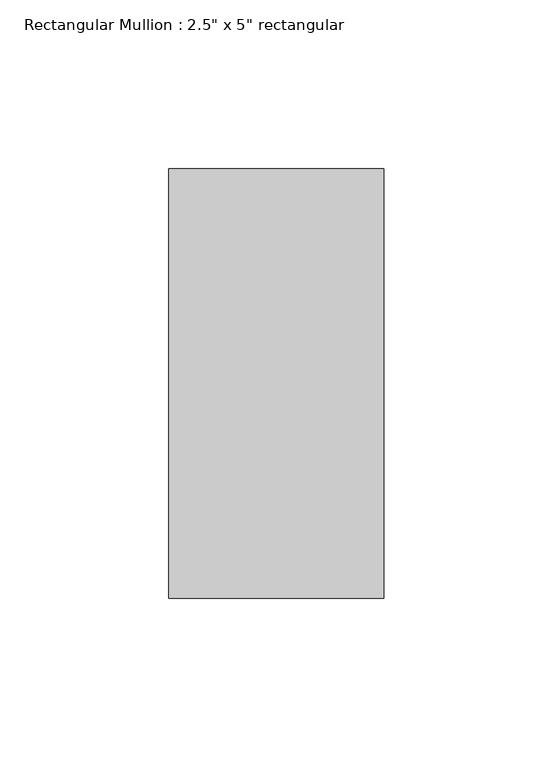
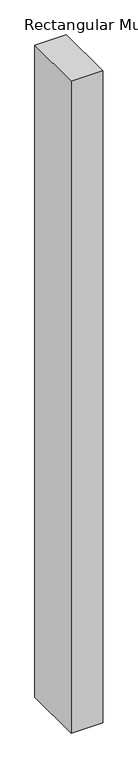
"""IFC4 building model written with IfcOpenShell, lengths in millimetres: member geometry."""

from ifc_helpers import new_model, si_unit, frame, origin, place, context, project, spatial, polyline, outline, extrude, source, transform, mapped, element, save


def member_4c2afa05(model_context):
    return source(origin(), model_context, "Body", "SweptSolid", [
        extrude(outline(polyline([(31.75, 63.5), (31.75, -63.5), (-31.75, -63.5), (-31.75, 63.5), (31.75, 63.5)])), frame((0.0, 0.0, -1391.4079139), z_axis=(0.0, 0.0, 1.0), x_axis=(1.0, 0.0, 0.0)), (0.0, 0.0, 1.0), 1391.4079139),
    ])


if __name__ == "__main__":
    model = new_model("IFC4")
    model_context = context("Model", 3, world=origin())
    ifc_project = project(units=[si_unit("LENGTHUNIT", "METRE", prefix="MILLI")], contexts=[model_context])
    site = spatial("IfcSite", under=ifc_project)
    building = spatial("IfcBuilding", under=site)
    placement = place(None, origin())
    member_shape = member_4c2afa05(model_context)
    element("IfcMember", 1, ObjectType="Rectangular Mullion : 2.5\" x 5\" rectangular", at=placement, inside=building, context=model_context, shape_type="MappedRepresentation", body=[
        mapped(member_shape, transform((0.0, 0.0, 0.0), x_axis=(1.0, 0.0, 0.0), y_axis=(0.0, 1.0, 0.0), z_axis=(0.0, 0.0, 1.0))),
    ])
    save(model, "model.ifc")

# Revit data of these elements
# Type "Rectangular Mullion : 2.5\" x 5\" rectangular"
#   built-in parameter 1007304 = 0.416667 (stored number, unit not read)
#   built-in parameter 1007301 = 0.104167 (stored number, unit not read)
#   built-in parameter 1007300 = 0.104167 (stored number, unit not read)
# Element 1 (IfcMember, "Rectangular Mullion : 2.5\" x 5\" rectangular")
#   Materials on its faces: "Aluminum"
# Materials
#   "Aluminum": class "Metal", colour RGB 247 247 247, transparency 0, Description = "Aluminum 6061", Cost = 0
